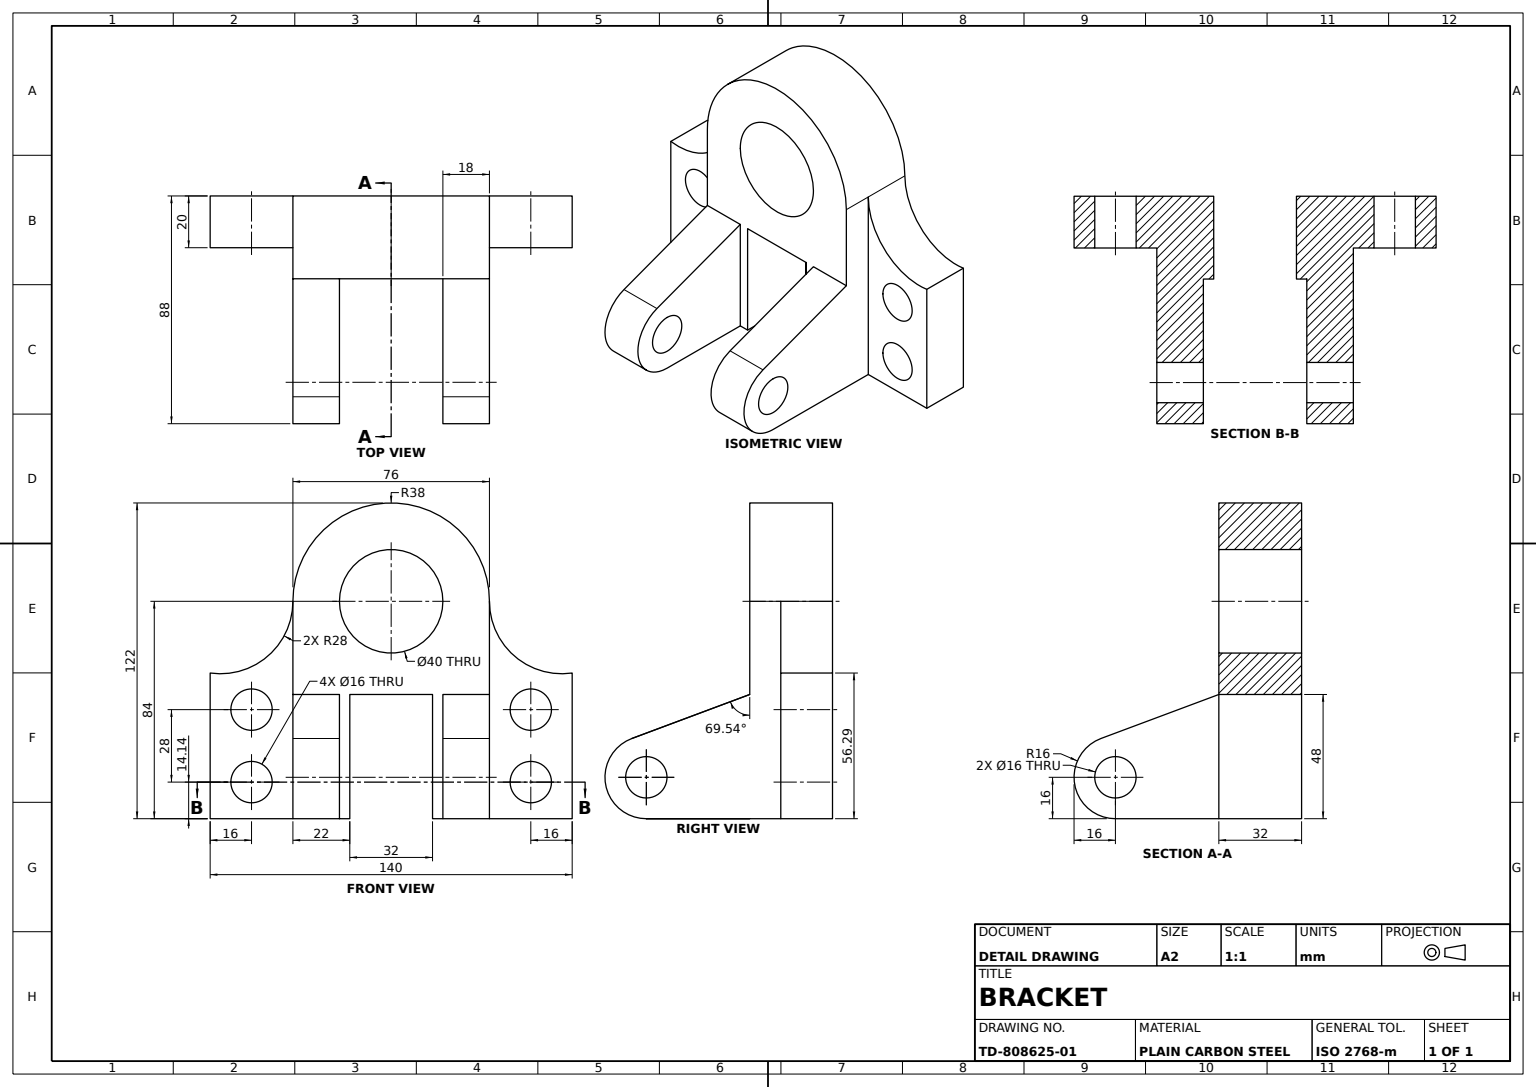
from build123d import *

# Parameters (mm, degrees)
BASE_BLOCK_DEPTH              = 32
FORK_ARMS_DEPTH               = 20
SIDE_FLANGE_DEPTH             = 18
FLANGE_START                  = -18
FLANGE_EXTENSION_DEPTH        = 18
FORK_SLOT_SKETCH_W            = 32
FORK_SLOT_SKETCH_H            = 48
FORK_SLOT_48X32_DEPTH         = 123.849501423
FORK_ARM_PROFILE_CUT_SKETCH_R = 8
FORK_ARM_PROFILE_CUT_DEPTH    = 129.763348823
FLANGE_HOLES_SKETCH_R         = 8
FLANGE_HOLES_16_DEPTH         = 163.677595261
PIVOT_BORE_SKETCH_R           = 20
PIVOT_BORE_40_DEPTH           = 123.849501423


with BuildPart() as part:
    # Base Block Sketch → Base Block (new body)
    with BuildSketch(Plane.XY):
        with BuildLine():
            Line((-38, 0), (-38, -84))
            Line((-38, -84), (38, -84))
            Line((38, -84), (38, 0))
            ThreePointArc((38, 0), (0, 38), (-38, 0))
        make_face()
    extrude(amount=BASE_BLOCK_DEPTH)

    # Fork Arms Sketch → Fork Arms (add)
    with BuildSketch(Plane(origin=(0, 0, 0), x_dir=(-1, 0, 0), z_dir=(0, 0, -1))):
        with BuildLine():
            Line((38, -84), (70, -84))
            Line((70, -84), (70, -27.712812921))
            ThreePointArc((70, -27.712812921), (47.66969722, -21.166010489), (38, 0))
            Line((38, 0), (38, -84))
        make_face()
        with BuildLine():
            Line((-38, -84), (-70, -84))
            Line((-70, -84), (-70, -27.712812921))
            ThreePointArc((-70, -27.712812921), (-47.66969722, -21.166010489), (-38, 0))
            Line((-38, 0), (-38, -84))
        make_face()
    extrude(amount=-FORK_ARMS_DEPTH)

    # Side Flange Sketch → Side Flange (add)
    with BuildSketch(Plane.ZY.offset(38)):
        with BuildLine():
            Line((72, -84), (32, -84))
            Line((32, -84), (32, -36))
            Line((32, -36), (77.592604925, -53.009243843))
            ThreePointArc((77.592604925, -53.009243843), (87.745667634, -70.841469822), (72, -84))
        make_face()
    extrude(amount=-SIDE_FLANGE_DEPTH)

    # Flange Extension Sketch → Flange Extension (add)
    with BuildSketch(Plane(origin=(38, 0, 0), x_dir=(0, 0, -1), z_dir=(1, 0, 0)).offset(FLANGE_START)):
        with BuildLine():
            Line((-72, -84), (-32, -84))
            Line((-32, -84), (-32, -36))
            Line((-32, -36), (-77.592604925, -53.009243843))
            ThreePointArc((-77.592604925, -53.009243843), (-87.745667634, -70.841469822), (-72, -84))
        make_face()
    extrude(amount=FLANGE_EXTENSION_DEPTH)

    # Fork Slot Sketch → Fork Slot 48x32 (cut, through all)
    with BuildSketch(Plane.XY.offset(32)):
        with Locations((0, -60)):
            Rectangle(FORK_SLOT_SKETCH_W, FORK_SLOT_SKETCH_H)
    extrude(amount=-FORK_SLOT_48X32_DEPTH, mode=Mode.SUBTRACT)

    # Fork Arm Profile Cut Sketch → Fork Arm Profile Cut (cut, through all)
    with BuildSketch(Plane.XY.offset(20)):
        with Locations((-54, -41.856406461)):
            Circle(FORK_ARM_PROFILE_CUT_SKETCH_R)
        with Locations((-54, -69.856406461)):
            Circle(FORK_ARM_PROFILE_CUT_SKETCH_R)
        with Locations((54, -41.856406461)):
            Circle(FORK_ARM_PROFILE_CUT_SKETCH_R)
        with Locations((54, -69.856406461)):
            Circle(FORK_ARM_PROFILE_CUT_SKETCH_R)
    extrude(amount=-FORK_ARM_PROFILE_CUT_DEPTH, mode=Mode.SUBTRACT)

    # Flange Holes Sketch → Flange Holes _16 (cut, through all)
    with BuildSketch(Plane.ZY.offset(38)):
        with Locations(Location((72, -68, 0), (0, 0, 270))):
            Circle(FLANGE_HOLES_SKETCH_R)
    extrude(amount=-FLANGE_HOLES_16_DEPTH, mode=Mode.SUBTRACT)

    # Pivot Bore Sketch → Pivot Bore _40 (cut, through all)
    with BuildSketch(Plane.XY.offset(32)):
        Circle(PIVOT_BORE_SKETCH_R)
    extrude(amount=-PIVOT_BORE_40_DEPTH, mode=Mode.SUBTRACT)


solid = part.part
